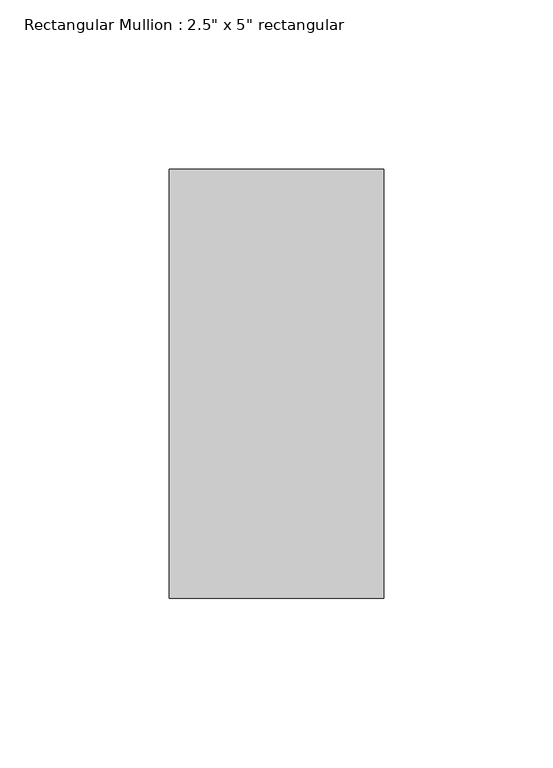
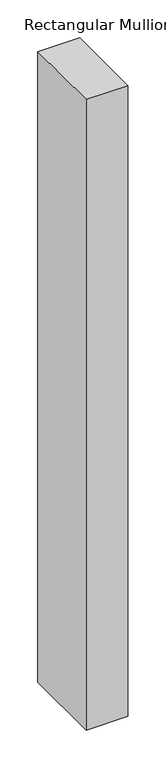
"""IFC4 building model written with IfcOpenShell, lengths in millimetres: member geometry."""

from ifc_helpers import new_model, si_unit, frame, origin, place, context, project, spatial, polyline, outline, extrude, source, transform, mapped, element, save


def member_f92b8aa2(model_context):
    return source(origin(), model_context, "Body", "SweptSolid", [
        extrude(outline(polyline([(31.75, 63.5), (31.75, -63.5), (-31.75, -63.5), (-31.75, 63.5), (31.75, 63.5)])), frame((0.0, 0.0, -1016.0), z_axis=(0.0, 0.0, 1.0), x_axis=(1.0, 0.0, 0.0)), (0.0, 0.0, 1.0), 1016.0),
    ])


if __name__ == "__main__":
    model = new_model("IFC4")
    model_context = context("Model", 3, world=origin())
    ifc_project = project(units=[si_unit("LENGTHUNIT", "METRE", prefix="MILLI")], contexts=[model_context])
    site = spatial("IfcSite", under=ifc_project)
    building = spatial("IfcBuilding", under=site)
    placement = place(None, origin())
    member_shape = member_f92b8aa2(model_context)
    element("IfcMember", 1, ObjectType="Rectangular Mullion : 2.5\" x 5\" rectangular", at=placement, inside=building, context=model_context, shape_type="MappedRepresentation", body=[
        mapped(member_shape, transform((0.0, 0.0, 0.0), x_axis=(1.0, 0.0, 0.0), y_axis=(0.0, 1.0, 0.0), z_axis=(0.0, 0.0, 1.0))),
    ])
    save(model, "model.ifc")

# Revit data of these elements
# Type "Rectangular Mullion : 2.5\" x 5\" rectangular"
#   built-in parameter 1007304 = 0.416667 (stored number, unit not read)
#   built-in parameter 1007301 = 0.104167 (stored number, unit not read)
#   built-in parameter 1007300 = 0.104167 (stored number, unit not read)
